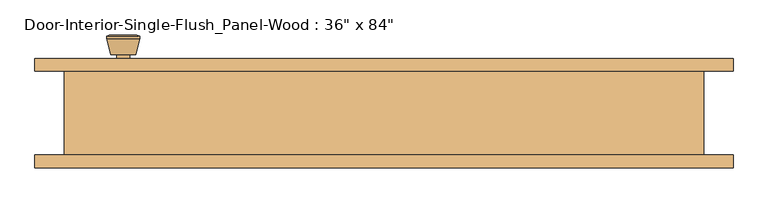
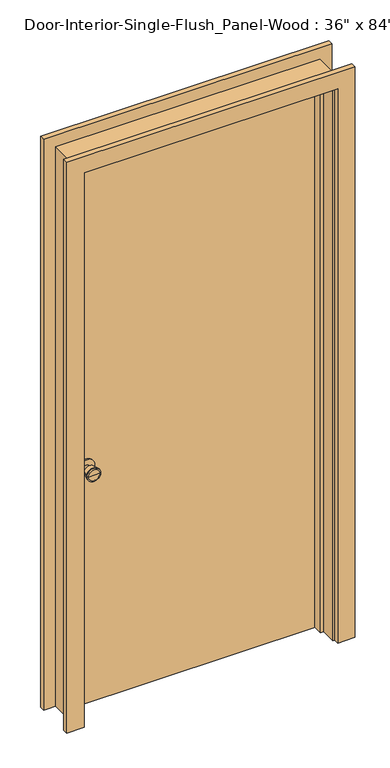
"""IFC4 building model written with IfcOpenShell, lengths in millimetres: door geometry."""

from ifc_helpers import new_model, si_unit, point, frame, frame_2d, origin, origin_with_axes, place, context, project, spatial, polyline, circle_curve, trimmed, segment, composite_curve, outline, extrude, faceted_brep, source, transform, mapped, element, save
from ifc_brep_helpers import plane_surface, cylinder_surface, revolved_surface, advanced_brep


def door_92402058(model_context):
    return source(origin(), model_context, "Body", "SolidModel", [
        advanced_brep(
        [(-393.7, 19.4, 914.4), (-383.7, 19.4, 914.4), (-403.7, 19.4, 914.4), (-373.2241324, -29.6, 914.4), (-393.7, -29.6, 914.4), (-414.1758676, -29.6, 914.4), (-368.7, -27.7721319, 914.4), (-418.7, -27.7721319, 914.4), (-368.7, -24.3084537, 914.4), (-418.7, -24.3084537, 914.4), (-375.063764, 0.4, 914.4), (-412.336236, 0.4, 914.4), (-383.7, 0.4, 914.4), (-403.7, 0.4, 914.4)],
        [
            (0, 1),
            (1, 2, circle_curve(frame((-393.7, 19.4, 914.4), z_axis=(0.0, 1.0, 0.0), x_axis=(-1.0, 0.0, 0.0)), 10.0)),
            (2, 0),
            (2, 1, circle_curve(frame((-393.7, 19.4, 914.4), z_axis=(0.0, 1.0, 0.0), x_axis=(-1.0, 0.0, 0.0)), 10.0)),
            (3, 4),
            (4, 5),
            (5, 3, circle_curve(frame((-393.7, -29.6, 914.4), z_axis=(0.0, -1.0, 0.0), x_axis=(-1.0, 0.0, 0.0)), 20.4758676)),
            (3, 5, circle_curve(frame((-393.7, -29.6, 914.4), z_axis=(0.0, -1.0, 0.0), x_axis=(-1.0, 0.0, 0.0)), 20.4758676)),
            (6, 3),
            (5, 7),
            (7, 6, circle_curve(frame((-393.7, -27.7721319, 914.4), z_axis=(0.0, -1.0, 0.0), x_axis=(-1.0, 0.0, 0.0)), 25.0)),
            (6, 7, circle_curve(frame((-393.7, -27.7721319, 914.4), z_axis=(0.0, -1.0, 0.0), x_axis=(-1.0, 0.0, 0.0)), 25.0)),
            (8, 6),
            (7, 9),
            (9, 8, circle_curve(frame((-393.7, -24.3084537, 914.4), z_axis=(0.0, -1.0, 0.0), x_axis=(-1.0, 0.0, 0.0)), 25.0)),
            (8, 9, circle_curve(frame((-393.7, -24.3084537, 914.4), z_axis=(0.0, -1.0, 0.0), x_axis=(-1.0, 0.0, 0.0)), 25.0)),
            (10, 8),
            (9, 11),
            (11, 10, circle_curve(frame((-393.7, 0.4, 914.4), z_axis=(0.0, -1.0, 0.0), x_axis=(-1.0, 0.0, 0.0)), 18.636236)),
            (10, 11, circle_curve(frame((-393.7, 0.4, 914.4), z_axis=(0.0, -1.0, 0.0), x_axis=(-1.0, 0.0, 0.0)), 18.636236)),
            (12, 10),
            (11, 13),
            (13, 12, circle_curve(frame((-393.7, 0.4, 914.4), z_axis=(0.0, -1.0, 0.0), x_axis=(-1.0, 0.0, 0.0)), 10.0)),
            (12, 13, circle_curve(frame((-393.7, 0.4, 914.4), z_axis=(0.0, -1.0, 0.0), x_axis=(-1.0, 0.0, 0.0)), 10.0)),
            (1, 12),
            (13, 2),
        ],
        [
            plane_surface(frame((-393.7, 19.4, 914.4), z_axis=(0.0, 1.0, 0.0), x_axis=(-1.0, 0.0, 0.0))),
            plane_surface(frame((-393.7, -29.6, 914.4), z_axis=(0.0, -1.0, 0.0), x_axis=(-1.0, 0.0, 0.0))),
            revolved_surface(polyline([(-414.1758676, -29.6, 914.4), (-418.7, -27.7721319, 914.4)]), (-393.7, 19.4, 914.4), (0.0, 1.0, 0.0)),
            cylinder_surface(frame((-393.7, 19.4, 914.4), z_axis=(0.0, 1.0, 0.0), x_axis=(-1.0, 0.0, 0.0)), 25.0),
            revolved_surface(polyline([(-418.7, -24.3084537, 914.4), (-412.336236, 0.4, 914.4)]), (-393.7, 19.4, 914.4), (0.0, 1.0, 0.0)),
            plane_surface(frame((-393.7, 0.4, 914.4), z_axis=(0.0, 1.0, 0.0), x_axis=(-1.0, 0.0, 0.0))),
            cylinder_surface(frame((-393.7, 19.4, 914.4), z_axis=(0.0, 1.0, 0.0), x_axis=(-1.0, 0.0, 0.0)), 10.0),
        ],
        [
            (0, [[1, 2, 3]]),
            (0, [[-3, 4, -1]]),
            (1, [[5, 6, 7]]),
            (1, [[-6, -5, 8]]),
            (2, [[9, -7, 10, 11]]),
            (2, [[-10, -8, -9, 12]]),
            (3, [[13, -11, 14, 15]]),
            (3, [[-14, -12, -13, 16]]),
            (4, [[17, -15, 18, 19]]),
            (4, [[-18, -16, -17, 20]]),
            (5, [[21, -19, 22, 23]]),
            (5, [[-22, -20, -21, 24]]),
            (6, [[25, -23, 26, -2]]),
            (6, [[-26, -24, -25, -4]]),
        ],
    ),
        extrude(outline(composite_curve([segment(trimmed(circle_curve(frame_2d((914.4, -393.7)), 30.0), [point((914.4, -423.7))], [point((914.4, -363.7))], False, "CARTESIAN"), True, "CONTINUOUS"), segment(trimmed(circle_curve(frame_2d((914.4, -393.7)), 30.0), [point((914.4, -363.7))], [point((914.4, -423.7))], False, "CARTESIAN"), True, "CONTINUOUS")], self_intersect=False)), frame((0.0, 19.4, 0.0), z_axis=(0.0, 1.0, 0.0), x_axis=(0.0, 0.0, 1.0)), (0.0, 0.0, 1.0), 6.0),
        advanced_brep(
        [(-393.7, 66.325, 914.4), (-403.7, 66.325, 914.4), (-383.7, 66.325, 914.4), (-373.2241324, 115.325, 914.4), (-414.1758676, 115.325, 914.4), (-393.7, 115.325, 914.4), (-368.7, 113.4971319, 914.4), (-418.7, 113.4971319, 914.4), (-368.7, 110.0334537, 914.4), (-418.7, 110.0334537, 914.4), (-375.063764, 85.325, 914.4), (-412.336236, 85.325, 914.4), (-383.7, 85.325, 914.4), (-403.7, 85.325, 914.4)],
        [
            (0, 1),
            (1, 2, circle_curve(frame((-393.7, 66.325, 914.4), z_axis=(0.0, -1.0, 0.0), x_axis=(-1.0, 0.0, 0.0)), 10.0)),
            (2, 0),
            (2, 1, circle_curve(frame((-393.7, 66.325, 914.4), z_axis=(0.0, -1.0, 0.0), x_axis=(-1.0, 0.0, 0.0)), 10.0)),
            (3, 4, circle_curve(frame((-393.7, 115.325, 914.4), z_axis=(0.0, 1.0, 0.0), x_axis=(-1.0, 0.0, 0.0)), 20.4758676)),
            (4, 5),
            (5, 3),
            (4, 3, circle_curve(frame((-393.7, 115.325, 914.4), z_axis=(0.0, 1.0, 0.0), x_axis=(-1.0, 0.0, 0.0)), 20.4758676)),
            (6, 7, circle_curve(frame((-393.7, 113.4971319, 914.4), z_axis=(0.0, 1.0, 0.0), x_axis=(-1.0, 0.0, 0.0)), 25.0)),
            (7, 4),
            (3, 6),
            (7, 6, circle_curve(frame((-393.7, 113.4971319, 914.4), z_axis=(0.0, 1.0, 0.0), x_axis=(-1.0, 0.0, 0.0)), 25.0)),
            (8, 9, circle_curve(frame((-393.7, 110.0334537, 914.4), z_axis=(0.0, 1.0, 0.0), x_axis=(-1.0, 0.0, 0.0)), 25.0)),
            (9, 7),
            (6, 8),
            (9, 8, circle_curve(frame((-393.7, 110.0334537, 914.4), z_axis=(0.0, 1.0, 0.0), x_axis=(-1.0, 0.0, 0.0)), 25.0)),
            (10, 11, circle_curve(frame((-393.7, 85.325, 914.4), z_axis=(0.0, 1.0, 0.0), x_axis=(-1.0, 0.0, 0.0)), 18.636236)),
            (11, 9),
            (8, 10),
            (11, 10, circle_curve(frame((-393.7, 85.325, 914.4), z_axis=(0.0, 1.0, 0.0), x_axis=(-1.0, 0.0, 0.0)), 18.636236)),
            (12, 13, circle_curve(frame((-393.7, 85.325, 914.4), z_axis=(0.0, 1.0, 0.0), x_axis=(-1.0, 0.0, 0.0)), 10.0)),
            (13, 11),
            (10, 12),
            (13, 12, circle_curve(frame((-393.7, 85.325, 914.4), z_axis=(0.0, 1.0, 0.0), x_axis=(-1.0, 0.0, 0.0)), 10.0)),
            (1, 13),
            (12, 2),
        ],
        [
            plane_surface(frame((-393.7, 66.325, 914.4), z_axis=(0.0, -1.0, 0.0), x_axis=(-1.0, 0.0, 0.0))),
            plane_surface(frame((-393.7, 115.325, 914.4), z_axis=(0.0, 1.0, 0.0), x_axis=(-1.0, 0.0, 0.0))),
            revolved_surface(polyline([(-414.1758676, 115.325, 914.4), (-418.7, 113.4971319, 914.4)]), (-393.7, 66.325, 914.4), (0.0, -1.0, 0.0)),
            cylinder_surface(frame((-393.7, 66.325, 914.4), z_axis=(0.0, -1.0, 0.0), x_axis=(-1.0, 0.0, 0.0)), 25.0),
            revolved_surface(polyline([(-418.7, 110.0334537, 914.4), (-412.336236, 85.325, 914.4)]), (-393.7, 66.325, 914.4), (0.0, -1.0, 0.0)),
            plane_surface(frame((-393.7, 85.325, 914.4), z_axis=(0.0, -1.0, 0.0), x_axis=(-1.0, 0.0, 0.0))),
            cylinder_surface(frame((-393.7, 66.325, 914.4), z_axis=(0.0, -1.0, 0.0), x_axis=(-1.0, 0.0, 0.0)), 10.0),
        ],
        [
            (0, [[1, 2, 3]]),
            (0, [[-3, 4, -1]]),
            (1, [[5, 6, 7]]),
            (1, [[8, -7, -6]]),
            (2, [[9, 10, -5, 11]]),
            (2, [[12, -11, -8, -10]]),
            (3, [[13, 14, -9, 15]]),
            (3, [[16, -15, -12, -14]]),
            (4, [[17, 18, -13, 19]]),
            (4, [[20, -19, -16, -18]]),
            (5, [[21, 22, -17, 23]]),
            (5, [[24, -23, -20, -22]]),
            (6, [[-2, 25, -21, 26]]),
            (6, [[-4, -26, -24, -25]]),
        ],
    ),
        extrude(outline(composite_curve([segment(trimmed(circle_curve(frame_2d((914.4, -393.7)), 30.0), [point((914.4, -423.7))], [point((914.4, -363.7))], False, "CARTESIAN"), True, "CONTINUOUS"), segment(trimmed(circle_curve(frame_2d((914.4, -393.7)), 30.0), [point((914.4, -363.7))], [point((914.4, -423.7))], False, "CARTESIAN"), True, "CONTINUOUS")], self_intersect=False)), frame((0.0, 60.325, 0.0), z_axis=(0.0, 1.0, 0.0), x_axis=(0.0, 0.0, 1.0)), (0.0, 0.0, 1.0), 6.0),
        faceted_brep([(482.6, 60.325, 0.0), (482.6, -66.675, 0.0), (457.2, -66.675, 0.0), (457.2, -9.525, 0.0), (444.5, -9.525, 0.0), (444.5, 25.4, 0.0), (457.2, 25.4, 0.0), (457.2, 60.325, 0.0), (482.6, 60.325, 2159.0), (482.6, -66.675, 2159.0), (-482.6, -66.675, 2159.0), (-482.6, -66.675, 0.0), (-457.2, -66.675, 0.0), (-457.2, -66.675, 2133.6), (457.2, -66.675, 2133.6), (457.2, -9.525, 2133.6), (-457.2, -9.525, 2133.6), (-457.2, -9.525, 0.0), (-444.5, -9.525, 0.0), (-444.5, -9.525, 2120.9), (444.5, -9.525, 2120.9), (444.5, 25.4, 2120.9), (-444.5, 25.4, 2120.9), (-444.5, 25.4, 0.0), (-457.2, 25.4, 0.0), (-457.2, 25.4, 2133.6), (457.2, 25.4, 2133.6), (457.2, 60.325, 2133.6), (-457.2, 60.325, 2133.6), (-457.2, 60.325, 0.0), (-482.6, 60.325, 0.0), (-482.6, 60.325, 2159.0)], [[[0, 1, 2, 3, 4, 5, 6, 7]], [[1, 0, 8, 9]], [[2, 1, 9, 10, 11, 12, 13, 14]], [[3, 2, 14, 15]], [[4, 3, 15, 16, 17, 18, 19, 20]], [[5, 4, 20, 21]], [[6, 5, 21, 22, 23, 24, 25, 26]], [[7, 6, 26, 27]], [[0, 7, 27, 28, 29, 30, 31, 8]], [[9, 8, 31, 10]], [[15, 14, 13, 16]], [[21, 20, 19, 22]], [[27, 26, 25, 28]], [[30, 29, 24, 23, 18, 17, 12, 11]], [[10, 31, 30, 11]], [[16, 13, 12, 17]], [[22, 19, 18, 23]], [[28, 25, 24, 29]]]),
        extrude(outline(polyline([(457.2, 25.4), (-457.2, 25.4), (-457.2, 60.325), (457.2, 60.325), (457.2, 25.4)])), origin_with_axes(), (0.0, 0.0, 1.0), 2133.6),
        extrude(outline(polyline([(0.0, 463.55), (0.0, 527.05), (2203.45, 527.05), (2203.45, -527.05), (0.0, -527.05), (0.0, -463.55), (2139.95, -463.55), (2139.95, 463.55), (0.0, 463.55)])), frame((0.0, 60.325, 0.0), z_axis=(0.0, 1.0, 0.0), x_axis=(0.0, 0.0, 1.0)), (0.0, 0.0, 1.0), 19.05),
        extrude(outline(polyline([(0.0, 463.55), (0.0, 527.05), (2203.45, 527.05), (2203.45, -527.05), (0.0, -527.05), (0.0, -463.55), (2139.95, -463.55), (2139.95, 463.55), (0.0, 463.55)])), frame((0.0, -85.725, 0.0), z_axis=(0.0, 1.0, 0.0), x_axis=(0.0, 0.0, 1.0)), (0.0, 0.0, 1.0), 19.05),
    ])


if __name__ == "__main__":
    model = new_model("IFC4")
    model_context = context("Model", 3, world=origin())
    ifc_project = project(units=[si_unit("LENGTHUNIT", "METRE", prefix="MILLI")], contexts=[model_context])
    site = spatial("IfcSite", under=ifc_project)
    building = spatial("IfcBuilding", under=site)
    placement = place(None, origin())
    door_shape = door_92402058(model_context)
    element("IfcDoor", 1, ObjectType="Door-Interior-Single-Flush_Panel-Wood : 36\" x 84\"", at=placement, inside=building, context=model_context, shape_type="MappedRepresentation", body=[
        mapped(door_shape, transform((0.0, 0.0, 0.0), x_axis=(1.0, 0.0, 0.0), y_axis=(0.0, 1.0, 0.0), z_axis=(0.0, 0.0, 1.0))),
    ])
    save(model, "model.ifc")

# Revit data of these elements
# Type "Door-Interior-Single-Flush_Panel-Wood : 36\" x 84\""
#   Type Mark = "8"
#   Assembly Code = "C1020300"
#   Analytic Construction = "Wooden"
#   Thickness = 0' - 1 3/8"
#   Thermal Resistance (R) = 2.5876 (h·ft²·°F)/BTU
#   Swing Angle [instance default] = 90.00°
#   Rough Width = 3' - 2"
#   Rough Height = 7' - 1"
#   Height = 7' - 0"
#   Width = 3' - 0"
#   Heat Transfer Coefficient (U) = 0.3865 BTU/(h·ft²·°F)
#   Trim Material = Cherry
#   Panel Material = Cherry
#   Frame Material = Cherry
#   Door Handle Material = Aluminum
#   Visual Light Transmittance = 0
#   Solar Heat Gain Coefficient = 0
#   Wall Closure = (empty or 0)
#   Function = (empty or 0)
# Element 1 (IfcDoor, "Door-Interior-Single-Flush_Panel-Wood : 36\" x 84\"")
#   Materials on its faces: "Cherry", "Aluminum"
# Materials
#   "Cherry": class "Wood", colour RGB 226 177 128, transparency 0, Description = "Prunus Serotina", Cost = 0
#   "Aluminum": class "Metal", colour RGB 247 247 247, transparency 0, Description = "Aluminum 6061", Cost = 0
